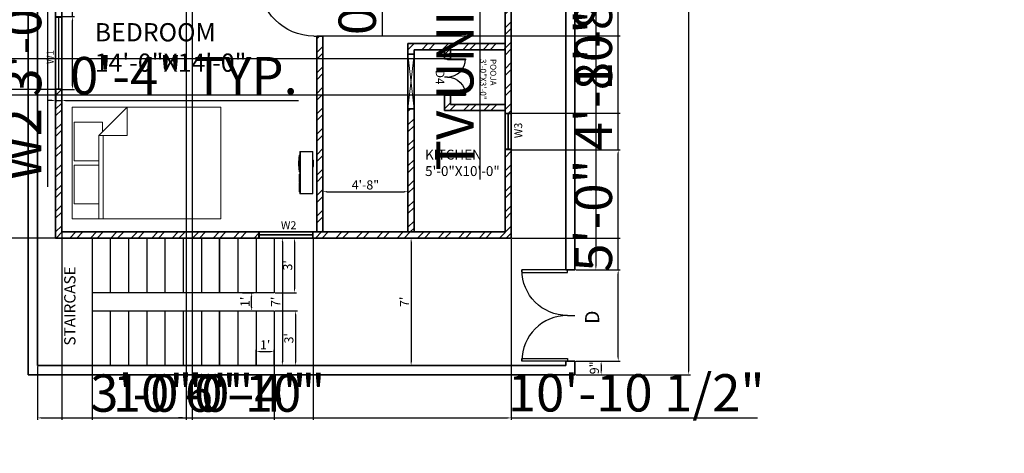
# Model space of a CAD drawing. Units: inches. Extents: x 1542 to 2523, y 1699 to 2449.
# Tile 2 of 7: x 1875 to 2523, y 1699 to 1984. Entities that reach past the tile are written whole.
import ezdxf

# ---------------------------------------------------------------- set-up
doc = ezdxf.new("R2010")
doc.units = ezdxf.units.IN
for name, color, linetype, lineweight in [('A-ANNO-DIMS', 7, 'Continuous', 18), ('A-ANNO-TEXT', 1, 'Continuous', 18), ('A-AREA-IDEN', 1, 'Continuous', 25), ('A-WALL-PATT', 9, 'Continuous', 13), ('doors', 5, 'Continuous', 25), ('furniture', 9, 'Continuous', 18), ('stair case', 6, 'Continuous', 25), ('walls', 7, 'Continuous', 35), ('windows', 93, 'Continuous', 18)]:
    doc.layers.add(name, color=color, linetype=linetype, lineweight=lineweight)
doc.styles.get("Standard").update_dxf_attribs({"font": 'arial.ttf'})
doc.dimstyles.new('ISO-25', dxfattribs={"dimtxt": 24.5625, "dimasz": 2.5, "dimexe": 1.25, "dimexo": 0.625, "dimtad": 1, "dimlunit": 4, "dimtxsty": 'Standard', "dimcen": 2.5, "dimadec": 0, "dimazin": 0, "dimtfac": 10, "dimtmove": 0, "dimatfit": 3, "dimfxl": 1, "dimarcsym": 0})

# ---------------------------------------------------------------- blocks, each defined once
blk = doc.blocks.new('*U2')
for p, q in [((0, 0), (0, -5)), ((30, 0), (30, -5))]:
    blk.add_line(p, q)
blk.add_lwpolyline([(0, 0), (0, 30), (1.75, 30), (1.75, 0)], close=True)
blk.add_arc((0, 0), 30, 0, 90)
blk = doc.blocks.new('Bed - Queen')
for p, q in [((0, -80.00003), (0, 0)), ((0, 0), (59.99999, 0)), ((59.99999, 0), (59.99999, -80.00003)), ((7.99999, -1.2), (28.79998, -1.2)), ((7.99999, -14.4), (7.99999, -1.2)), ((28.79998, -1.2), (28.79998, -14.4)), ((31.19999, -1.2), (51.99999, -1.2)), ((31.19999, -14.4), (31.19999, -1.2)), ((51.99999, -1.2), (51.99999, -16.4)), ((0, -14.4), (44.8, -14.4)), ((59.99999, -29.6), (44.8, -14.4)), ((44.8, -14.4), (44.8, -29.6)), ((44.8, -16.8), (0, -16.8)), ((51.99999, -16.4), (46.79936, -16.4)), ((44.8, -29.6), (59.99999, -29.6)), ((59.99999, -80.00003), (0, -80.00003))]:
    blk.add_line(p, q)
blk = doc.blocks.new('Entertainment Center')
for p, q in [((-4, 0), (-5, -1)), ((4, 0), (-4, 0)), ((5, -1), (4, 0)), ((-17, -19), (-17, -1)), ((-17, -1), (43, -1)), ((-16.5, -18.5), (-16.5, -1.5)), ((-16.5, -1.5), (42.5, -1.5)), ((42.5, -1.5), (42.5, -18.5)), ((43, -1), (43, -19)), ((43, -19), (-17, -19)), ((42.5, -18.5), (-16.5, -18.5)), ((-12, -20), (-12, -19)), ((12, -20), (-12, -20)), ((12, -19), (12, -20)), ((15, -20), (15, -19)), ((27, -20), (15, -20)), ((27, -19), (27, -20)), ((28, -20), (28, -19)), ((40, -20), (28, -20)), ((40, -19), (40, -20))]:
    blk.add_line(p, q)
blk.add_arc((0, 40), 61, 259.6111, 280.3889)
blk = doc.blocks.new('*D10')
at = {"layer": 'A-ANNO-DIMS', "color": 0, "lineweight": -2, "transparency": 16777216}
for p, q in [((2241.01, 2290.44), (2316.46, 2290.44)), ((2315.21, 2287.94), (2315.21, 1752.94)), ((2241.01, 1750.44), (2316.46, 1750.44))]:
    blk.add_line(p, q, dxfattribs=at)
at = {"layer": 'A-ANNO-DIMS', "color": 0, "transparency": 16777216}
for points in [[(2314.79, 2287.94), (2315.62, 2287.94), (2315.21, 2290.44)], [(2314.79, 1752.94), (2315.62, 1752.94), (2315.21, 1750.44)]]:
    blk.add_solid(points, dxfattribs=at)
at = {"layer": 'Defpoints', "color": 0, "transparency": 16777216}
for p in [(2240.38, 2290.44), (2240.38, 1750.44), (2315.21, 1750.44)]:
    blk.add_point(p, dxfattribs=at)
at = {"layer": 'A-ANNO-DIMS', "color": 0, "transparency": 16777216, "insert": (2308.48, 2020.44), "char_height": 12, "attachment_point": 5, "rotation": 90}
blk.add_mtext("45'", dxfattribs=at)
blk = doc.blocks.new('*D11')
at = {"layer": 'A-ANNO-DIMS', "color": 0, "lineweight": -2, "transparency": 16777216}
for p, q in [((2241.01, 2290.44), (2255.4, 2290.44)), ((2254.15, 2287.94), (2254.15, 1821.94)), ((2241.01, 1819.44), (2255.4, 1819.44))]:
    blk.add_line(p, q, dxfattribs=at)
at = {"layer": 'A-ANNO-DIMS', "color": 0, "transparency": 16777216}
for points in [[(2253.73, 2287.94), (2254.57, 2287.94), (2254.15, 2290.44)], [(2253.73, 1821.94), (2254.57, 1821.94), (2254.15, 1819.44)]]:
    blk.add_solid(points, dxfattribs=at)
at = {"layer": 'Defpoints', "color": 0, "transparency": 16777216}
for p in [(2240.38, 2290.44), (2240.38, 1819.44), (2254.15, 1819.44)]:
    blk.add_point(p, dxfattribs=at)
at = {"layer": 'A-ANNO-DIMS', "color": 0, "transparency": 16777216, "insert": (2250.46, 2054.94), "char_height": 6, "attachment_point": 5, "rotation": 90}
blk.add_mtext('39\'-3"', dxfattribs=at)
blk = doc.blocks.new('*D14')
at = {"layer": 'A-ANNO-DIMS', "color": 0, "lineweight": -2, "transparency": 16777216}
for p, q in [((2030.38, 1757.06), (2030.38, 1766.92)), ((2032.88, 1765.67), (2039.88, 1765.67)), ((2042.38, 1757.06), (2042.38, 1766.92))]:
    blk.add_line(p, q, dxfattribs=at)
at = {"layer": 'A-ANNO-DIMS', "color": 0, "transparency": 16777216}
for points in [[(2032.88, 1766.08), (2032.88, 1765.25), (2030.38, 1765.67)], [(2039.88, 1766.08), (2039.88, 1765.25), (2042.38, 1765.67)]]:
    blk.add_solid(points, dxfattribs=at)
at = {"layer": 'Defpoints', "color": 0, "transparency": 16777216}
for p in [(2042.38, 1765.67), (2030.38, 1756.44), (2042.38, 1756.44)]:
    blk.add_point(p, dxfattribs=at)
at = {"layer": 'A-ANNO-DIMS', "color": 0, "transparency": 16777216, "insert": (2036.38, 1769.3), "char_height": 6, "attachment_point": 5}
blk.add_mtext("1'", dxfattribs=at)
blk = doc.blocks.new('*D15')
at = {"layer": 'A-ANNO-DIMS', "color": 0, "lineweight": -2, "transparency": 16777216}
for p, q in [((2043.01, 1840.44), (2056.9, 1840.44)), ((2055.65, 1837.94), (2055.65, 1806.94)), ((2043.01, 1804.44), (2056.9, 1804.44))]:
    blk.add_line(p, q, dxfattribs=at)
at = {"layer": 'A-ANNO-DIMS', "color": 0, "transparency": 16777216}
for points in [[(2055.24, 1837.94), (2056.07, 1837.94), (2055.65, 1840.44)], [(2055.24, 1806.94), (2056.07, 1806.94), (2055.65, 1804.44)]]:
    blk.add_solid(points, dxfattribs=at)
at = {"layer": 'Defpoints', "color": 0, "transparency": 16777216}
for p in [(2042.38, 1840.44), (2042.38, 1804.44), (2055.65, 1804.44)]:
    blk.add_point(p, dxfattribs=at)
at = {"layer": 'A-ANNO-DIMS', "color": 0, "transparency": 16777216, "insert": (2051.96, 1822.44), "char_height": 6, "attachment_point": 5, "rotation": 90}
blk.add_mtext("3'", dxfattribs=at)
blk = doc.blocks.new('*D16')
at = {"layer": 'A-ANNO-DIMS', "color": 0, "lineweight": -2, "transparency": 16777216}
for p, q in [((2128.01, 1840.44), (2133.74, 1840.44)), ((2132.49, 1837.94), (2132.49, 1758.94)), ((2128.01, 1756.44), (2133.74, 1756.44))]:
    blk.add_line(p, q, dxfattribs=at)
at = {"layer": 'A-ANNO-DIMS', "color": 0, "transparency": 16777216}
for points in [[(2132.07, 1837.94), (2132.9, 1837.94), (2132.49, 1840.44)], [(2132.07, 1758.94), (2132.9, 1758.94), (2132.49, 1756.44)]]:
    blk.add_solid(points, dxfattribs=at)
at = {"layer": 'Defpoints', "color": 0, "transparency": 16777216}
for p in [(2127.38, 1840.44), (2127.38, 1756.44), (2132.49, 1756.44)]:
    blk.add_point(p, dxfattribs=at)
at = {"layer": 'A-ANNO-DIMS', "color": 0, "transparency": 16777216, "insert": (2128.86, 1798.44), "char_height": 6, "attachment_point": 5, "rotation": 90}
blk.add_mtext("7'", dxfattribs=at)
blk = doc.blocks.new('*D18')
at = {"layer": 'A-ANNO-DIMS', "color": 0, "lineweight": -2, "transparency": 16777216}
for p, q in [((2043.01, 1840.44), (2048.95, 1840.44)), ((2047.7, 1837.94), (2047.7, 1758.94)), ((2043.01, 1756.44), (2048.95, 1756.44))]:
    blk.add_line(p, q, dxfattribs=at)
at = {"layer": 'A-ANNO-DIMS', "color": 0, "transparency": 16777216}
for points in [[(2047.28, 1837.94), (2048.11, 1837.94), (2047.7, 1840.44)], [(2047.28, 1758.94), (2048.11, 1758.94), (2047.7, 1756.44)]]:
    blk.add_solid(points, dxfattribs=at)
at = {"layer": 'Defpoints', "color": 0, "transparency": 16777216}
for p in [(2042.38, 1840.44), (2042.38, 1756.44), (2047.7, 1756.44)]:
    blk.add_point(p, dxfattribs=at)
at = {"layer": 'A-ANNO-DIMS', "color": 0, "transparency": 16777216, "insert": (2044.07, 1798.44), "char_height": 6, "attachment_point": 5, "rotation": 90}
blk.add_mtext("7'", dxfattribs=at)
blk = doc.blocks.new('*D19')
at = {"layer": 'A-ANNO-DIMS', "color": 0, "lineweight": -2, "transparency": 16777216}
for p, q in [((2043.01, 1792.44), (2057.68, 1792.44)), ((2056.43, 1789.94), (2056.43, 1758.94)), ((2043.01, 1756.44), (2057.68, 1756.44))]:
    blk.add_line(p, q, dxfattribs=at)
at = {"layer": 'A-ANNO-DIMS', "color": 0, "transparency": 16777216}
for points in [[(2056.01, 1789.94), (2056.84, 1789.94), (2056.43, 1792.44)], [(2056.01, 1758.94), (2056.84, 1758.94), (2056.43, 1756.44)]]:
    blk.add_solid(points, dxfattribs=at)
at = {"layer": 'Defpoints', "color": 0, "transparency": 16777216}
for p in [(2042.38, 1792.44), (2042.38, 1756.44), (2056.43, 1756.44)]:
    blk.add_point(p, dxfattribs=at)
at = {"layer": 'A-ANNO-DIMS', "color": 0, "transparency": 16777216, "insert": (2052.74, 1774.44), "char_height": 6, "attachment_point": 5, "rotation": 90}
blk.add_mtext("3'", dxfattribs=at)
blk = doc.blocks.new('*D20')
at = {"layer": 'A-ANNO-DIMS', "color": 0, "lineweight": -2, "transparency": 16777216}
for p, q in [((2021.4, 1804.44), (2028.73, 1804.44)), ((2027.48, 1794.94), (2027.48, 1801.94)), ((2021.4, 1792.44), (2028.73, 1792.44))]:
    blk.add_line(p, q, dxfattribs=at)
at = {"layer": 'A-ANNO-DIMS', "color": 0, "transparency": 16777216}
for points in [[(2027.06, 1801.94), (2027.9, 1801.94), (2027.48, 1804.44)], [(2027.06, 1794.94), (2027.9, 1794.94), (2027.48, 1792.44)]]:
    blk.add_solid(points, dxfattribs=at)
at = {"layer": 'Defpoints', "color": 0, "transparency": 16777216}
for p in [(2020.78, 1804.44), (2027.48, 1804.44), (2020.78, 1792.44)]:
    blk.add_point(p, dxfattribs=at)
at = {"layer": 'A-ANNO-DIMS', "color": 0, "transparency": 16777216, "insert": (2023.84, 1798.44), "char_height": 6, "attachment_point": 5, "rotation": 90}
blk.add_mtext("1'", dxfattribs=at)
blk = doc.blocks.new('*D21')
at = {"layer": 'A-ANNO-DIMS', "color": 0, "lineweight": -2, "transparency": 16777216}
for p, q in [((2074.38, 1858.36), (2074.38, 1872.17)), ((2076.88, 1870.92), (2127.88, 1870.92)), ((2130.38, 1858.36), (2130.38, 1872.17))]:
    blk.add_line(p, q, dxfattribs=at)
at = {"layer": 'A-ANNO-DIMS', "color": 0, "transparency": 16777216}
for points in [[(2076.88, 1871.34), (2076.88, 1870.5), (2074.38, 1870.92)], [(2127.88, 1871.34), (2127.88, 1870.5), (2130.38, 1870.92)]]:
    blk.add_solid(points, dxfattribs=at)
at = {"layer": 'Defpoints', "color": 0, "transparency": 16777216}
for p in [(2130.38, 1870.92), (2074.38, 1857.74), (2130.38, 1857.74)]:
    blk.add_point(p, dxfattribs=at)
at = {"layer": 'A-ANNO-DIMS', "color": 0, "transparency": 16777216, "insert": (2102.38, 1874.61), "char_height": 6, "attachment_point": 5}
blk.add_mtext('4\'-8"', dxfattribs=at)
blk = doc.blocks.new('*D22')
at = {"layer": 'A-ANNO-DIMS', "color": 0, "lineweight": -2, "transparency": 16777216}
for p, q in [((2241.01, 1759.44), (2258.85, 1759.44)), ((2257.6, 1756.94), (2257.6, 1752.94)), ((2241.01, 1750.44), (2258.85, 1750.44))]:
    blk.add_line(p, q, dxfattribs=at)
at = {"layer": 'A-ANNO-DIMS', "color": 0, "transparency": 16777216}
for points in [[(2257.18, 1756.94), (2258.02, 1756.94), (2257.6, 1759.44)], [(2257.18, 1752.94), (2258.02, 1752.94), (2257.6, 1750.44)]]:
    blk.add_solid(points, dxfattribs=at)
at = {"layer": 'Defpoints', "color": 0, "transparency": 16777216}
for p in [(2240.38, 1759.44), (2240.38, 1750.44), (2257.6, 1750.44)]:
    blk.add_point(p, dxfattribs=at)
at = {"layer": 'A-ANNO-DIMS', "color": 0, "transparency": 16777216, "insert": (2253.91, 1754.94), "char_height": 6, "attachment_point": 5, "rotation": 90}
blk.add_mtext('9"', dxfattribs=at)
blk = doc.blocks.new('WIN-W3-24IN')
for p, q in [((0, 0), (0, 24.03)), ((0, 24.03), (3.94, 24.03)), ((0, 23.53), (3.94, 23.53)), ((1.77, 0.5), (1.77, 23.53)), ((2.17, 0.5), (2.17, 23.53)), ((3.94, 24.03), (3.94, 0)), ((3.94, 0.5), (0, 0.5)), ((3.94, 0), (0, 0))]:
    blk.add_line(p, q)
blk = doc.blocks.new('WIN-W2-36IN')
for p, q in [((0, 3.94), (36.03, 3.94)), ((0, 0), (0, 3.94)), ((36.03, 0), (0, 0)), ((0.5, 0), (0.5, 3.94)), ((0.5, 2.17), (35.53, 2.17)), ((0.5, 1.77), (35.53, 1.77)), ((35.53, 3.94), (35.53, 0)), ((36.03, 3.94), (36.03, 0))]:
    blk.add_line(p, q)
blk = doc.blocks.new('WIN-W1-48IN')
for p, q in [((0, 0), (0, 48.03)), ((0, 48.03), (3.94, 48.03)), ((0, 47.53), (3.94, 47.53)), ((1.77, 0.5), (1.77, 47.53)), ((2.17, 0.5), (2.17, 47.53)), ((3.94, 48.03), (3.94, 0)), ((3.94, 0.5), (0, 0.5)), ((3.94, 0), (0, 0))]:
    blk.add_line(p, q)
blk = doc.blocks.new('*D27')
at = {"layer": 'A-ANNO-DIMS', "color": 0, "lineweight": -2, "transparency": 16777216}
for p, q in [((2114.72, 2156.7), (2112.11, 2156.7)), ((2113.36, 2154.2), (2113.36, 2148.3)), ((2114.72, 2145.8), (2112.11, 2145.8)), ((2113.36, 2145.8), (2113.36, 1973.25))]:
    blk.add_line(p, q, dxfattribs=at)
at = {"layer": 'A-ANNO-DIMS', "color": 0, "transparency": 16777216}
for points in [[(2112.94, 2154.2), (2113.78, 2154.2), (2113.36, 2156.7)], [(2112.94, 2148.3), (2113.78, 2148.3), (2113.36, 2145.8)]]:
    blk.add_solid(points, dxfattribs=at)
at = {"layer": 'Defpoints', "color": 0, "transparency": 16777216}
for p in [(2115.34, 2156.7), (2113.36, 2145.8), (2115.34, 2145.8)]:
    blk.add_point(p, dxfattribs=at)
at = {"layer": 'A-ANNO-DIMS', "color": 0, "transparency": 16777216, "insert": (2100.19, 2058.28), "char_height": 24.5625, "attachment_point": 5, "rotation": 90}
blk.add_mtext('0\'-11" TYP.', dxfattribs=at)
blk = doc.blocks.new('*D30')
at = {"layer": 'A-ANNO-DIMS', "color": 0, "lineweight": -2, "transparency": 16777216}
for p, q in [((2181.19, 2203.89), (2176.38, 2203.89)), ((2177.63, 2201.39), (2177.63, 2178.49)), ((2181.19, 2175.99), (2176.38, 2175.99)), ((2177.63, 2175.99), (2177.63, 1878.93))]:
    blk.add_line(p, q, dxfattribs=at)
at = {"layer": 'A-ANNO-DIMS', "color": 0, "transparency": 16777216}
for points in [[(2177.21, 2201.39), (2178.05, 2201.39), (2177.63, 2203.89)], [(2177.21, 2178.49), (2178.05, 2178.49), (2177.63, 2175.99)]]:
    blk.add_solid(points, dxfattribs=at)
at = {"layer": 'Defpoints', "color": 0, "transparency": 16777216}
for p in [(2181.81, 2203.89), (2177.63, 2175.99), (2181.81, 2175.99)]:
    blk.add_point(p, dxfattribs=at)
at = {"layer": 'A-ANNO-DIMS', "color": 0, "transparency": 16777216, "insert": (2164.46, 2026.21), "char_height": 24.5625, "attachment_point": 5, "rotation": 90}
blk.add_mtext('TV UNIT 2\'-4" TYP.', dxfattribs=at)
blk = doc.blocks.new('*D36')
at = {"layer": 'A-ANNO-DIMS', "color": 0, "lineweight": -2, "transparency": 16777216}
for p, q in [((1897.82, 2125.68), (1891.79, 2125.68)), ((1893.04, 2123.18), (1893.04, 2092.15)), ((1897.82, 2089.65), (1891.79, 2089.65)), ((1893.04, 2089.65), (1893.04, 1874.17))]:
    blk.add_line(p, q, dxfattribs=at)
at = {"layer": 'A-ANNO-DIMS', "color": 0, "transparency": 16777216}
for points in [[(1892.62, 2123.18), (1893.46, 2123.18), (1893.04, 2125.68)], [(1892.62, 2092.15), (1893.46, 2092.15), (1893.04, 2089.65)]]:
    blk.add_solid(points, dxfattribs=at)
at = {"layer": 'Defpoints', "color": 0, "transparency": 16777216}
for p in [(1898.45, 2125.68), (1893.04, 2089.65), (1898.45, 2089.65)]:
    blk.add_point(p, dxfattribs=at)
at = {"layer": 'A-ANNO-DIMS', "color": 0, "transparency": 16777216, "insert": (1879.87, 1980.66), "char_height": 24.5625, "attachment_point": 5, "rotation": 90}
blk.add_mtext('W2 3\'-0" TYP.', dxfattribs=at)
blk = doc.blocks.new('*D40')
at = {"layer": 'A-ANNO-DIMS', "color": 0, "lineweight": -2, "transparency": 16777216}
for p, q in [((1909.59, 1986.22), (1909.59, 2201.7)), ((1903.01, 1986.22), (1910.84, 1986.22)), ((1909.59, 1940.69), (1909.59, 1983.72)), ((1903.01, 1938.19), (1910.84, 1938.19))]:
    blk.add_line(p, q, dxfattribs=at)
at = {"layer": 'A-ANNO-DIMS', "color": 0, "transparency": 16777216}
for points in [[(1909.17, 1983.72), (1910, 1983.72), (1909.59, 1986.22)], [(1909.17, 1940.69), (1910, 1940.69), (1909.59, 1938.19)]]:
    blk.add_solid(points, dxfattribs=at)
at = {"layer": 'Defpoints', "color": 0, "transparency": 16777216}
for p in [(1902.38, 1986.22), (1909.59, 1986.22), (1902.38, 1938.19)]:
    blk.add_point(p, dxfattribs=at)
at = {"layer": 'A-ANNO-DIMS', "color": 0, "transparency": 16777216, "insert": (1896.42, 2095.21), "char_height": 24.5625, "attachment_point": 5, "rotation": 90}
blk.add_mtext('W1 4\'-0" TYP.', dxfattribs=at)
blk = doc.blocks.new('*D41')
at = {"layer": 'A-ANNO-DIMS', "color": 0, "lineweight": -2, "transparency": 16777216}
for p, q in [((1898.45, 1937.57), (1898.45, 1929.74)), ((1902.38, 1937.57), (1902.38, 1929.74)), ((1895.95, 1930.99), (1893.45, 1930.99)), ((1898.45, 1930.99), (1902.38, 1930.99)), ((1904.88, 1930.99), (2058.35, 1930.99))]:
    blk.add_line(p, q, dxfattribs=at)
at = {"layer": 'A-ANNO-DIMS', "color": 0, "transparency": 16777216}
for points in [[(1895.95, 1931.4), (1895.95, 1930.57), (1898.45, 1930.99)], [(1904.88, 1931.4), (1904.88, 1930.57), (1902.38, 1930.99)]]:
    blk.add_solid(points, dxfattribs=at)
at = {"layer": 'Defpoints', "color": 0, "transparency": 16777216}
for p in [(1898.45, 1938.19), (1902.38, 1938.19), (1902.38, 1930.99)]:
    blk.add_point(p, dxfattribs=at)
at = {"layer": 'A-ANNO-DIMS', "color": 0, "transparency": 16777216, "insert": (1982.87, 1944.15), "char_height": 24.562, "attachment_point": 5}
blk.add_mtext('0\'-4" TYP.', dxfattribs=at)
blk = doc.blocks.new('*D42')
at = {"layer": 'A-ANNO-DIMS', "color": 0, "lineweight": -2, "transparency": 16777216}
for p, q in [((2131.75, 2027.78), (2131.75, 2037.46)), ((2134.25, 2036.21), (2189.62, 2036.21)), ((2192.12, 2027.78), (2192.12, 2037.46)), ((2192.12, 2036.21), (2523.07, 2036.21))]:
    blk.add_line(p, q, dxfattribs=at)
at = {"layer": 'A-ANNO-DIMS', "color": 0, "transparency": 16777216}
for points in [[(2134.25, 2036.63), (2134.25, 2035.8), (2131.75, 2036.21)], [(2189.62, 2036.63), (2189.62, 2035.8), (2192.12, 2036.21)]]:
    blk.add_solid(points, dxfattribs=at)
at = {"layer": 'Defpoints', "color": 0, "transparency": 16777216}
for p in [(2192.12, 2036.21), (2131.75, 2027.16), (2192.12, 2027.16)]:
    blk.add_point(p, dxfattribs=at)
at = {"layer": 'A-ANNO-DIMS', "color": 0, "transparency": 16777216, "insert": (2358.84, 2049.54), "char_height": 24.5625, "attachment_point": 5}
blk.add_mtext('DINING SET 5\'-0 1/2"', dxfattribs=at)
blk = doc.blocks.new('*D47')
at = {"layer": 'A-ANNO-DIMS', "color": 0, "lineweight": -2, "transparency": 16777216}
for p, q in [((2268.83, 2009.44), (2268.83, 2078.47)), ((2071.01, 2009.44), (2270.08, 2009.44)), ((2268.83, 1975.94), (2268.83, 2006.94)), ((2071.01, 1973.44), (2270.08, 1973.44))]:
    blk.add_line(p, q, dxfattribs=at)
at = {"layer": 'A-ANNO-DIMS', "color": 0, "transparency": 16777216}
for points in [[(2268.42, 2006.94), (2269.25, 2006.94), (2268.83, 2009.44)], [(2268.42, 1975.94), (2269.25, 1975.94), (2268.83, 1973.44)]]:
    blk.add_solid(points, dxfattribs=at)
at = {"layer": 'Defpoints', "color": 0, "transparency": 16777216}
for p in [(2070.38, 2009.44), (2268.83, 2009.44), (2070.38, 1973.44)]:
    blk.add_point(p, dxfattribs=at)
at = {"layer": 'A-ANNO-DIMS', "color": 0, "transparency": 16777216, "insert": (2255.66, 2045.2), "char_height": 24.562, "attachment_point": 5, "rotation": 90}
blk.add_mtext('3\'-0"', dxfattribs=at)
blk = doc.blocks.new('*D49')
at = {"layer": 'A-ANNO-DIMS', "color": 0, "lineweight": -2, "transparency": 16777216}
for p, q in [((1851.93, 1958.44), (1851.93, 2027.9)), ((2157.76, 1958.44), (1850.68, 1958.44)), ((1851.93, 1936.94), (1851.93, 1955.94)), ((2157.76, 1934.44), (1850.68, 1934.44))]:
    blk.add_line(p, q, dxfattribs=at)
at = {"layer": 'A-ANNO-DIMS', "color": 0, "transparency": 16777216}
for points in [[(1851.52, 1955.94), (1852.35, 1955.94), (1851.93, 1958.44)], [(1851.52, 1936.94), (1852.35, 1936.94), (1851.93, 1934.44)]]:
    blk.add_solid(points, dxfattribs=at)
at = {"layer": 'Defpoints', "color": 0, "transparency": 16777216}
for p in [(1851.93, 1958.44), (2158.38, 1958.44), (2158.38, 1934.44)]:
    blk.add_point(p, dxfattribs=at)
at = {"layer": 'A-ANNO-DIMS', "color": 0, "transparency": 16777216, "insert": (1838.77, 1994.42), "char_height": 24.562, "attachment_point": 5, "rotation": 90}
blk.add_mtext('2\'-0"', dxfattribs=at)
blk = doc.blocks.new('*D51')
at = {"layer": 'A-ANNO-DIMS', "color": 0, "lineweight": -2, "transparency": 16777216}
for p, q in [((2268.83, 1819.44), (2268.83, 1888.48)), ((2241.01, 1819.44), (2270.08, 1819.44)), ((2268.83, 1761.94), (2268.83, 1816.94)), ((2241.01, 1759.44), (2270.08, 1759.44))]:
    blk.add_line(p, q, dxfattribs=at)
at = {"layer": 'A-ANNO-DIMS', "color": 0, "transparency": 16777216}
for points in [[(2268.42, 1816.94), (2269.25, 1816.94), (2268.83, 1819.44)], [(2268.42, 1761.94), (2269.25, 1761.94), (2268.83, 1759.44)]]:
    blk.add_solid(points, dxfattribs=at)
at = {"layer": 'Defpoints', "color": 0, "transparency": 16777216}
for p in [(2240.38, 1819.44), (2268.83, 1819.44), (2240.38, 1759.44)]:
    blk.add_point(p, dxfattribs=at)
at = {"layer": 'A-ANNO-DIMS', "color": 0, "transparency": 16777216, "insert": (2255.67, 1855.21), "char_height": 24.562, "attachment_point": 5, "rotation": 90}
blk.add_mtext('5\'-0"', dxfattribs=at)
blk = doc.blocks.new('*D52')
at = {"layer": 'A-ANNO-DIMS', "color": 0, "lineweight": -2, "transparency": 16777216}
for p, q in [((1886.38, 1755.81), (1886.38, 1720.74)), ((1922.38, 1755.81), (1922.38, 1720.74)), ((1888.88, 1721.99), (1919.88, 1721.99)), ((1922.38, 1721.99), (1991.41, 1721.99))]:
    blk.add_line(p, q, dxfattribs=at)
at = {"layer": 'A-ANNO-DIMS', "color": 0, "transparency": 16777216}
for points in [[(1888.88, 1722.41), (1888.88, 1721.57), (1886.38, 1721.99)], [(1919.88, 1722.41), (1919.88, 1721.57), (1922.38, 1721.99)]]:
    blk.add_solid(points, dxfattribs=at)
at = {"layer": 'Defpoints', "color": 0, "transparency": 16777216}
for p in [(1886.38, 1756.44), (1922.38, 1756.44), (1922.38, 1721.99)]:
    blk.add_point(p, dxfattribs=at)
at = {"layer": 'A-ANNO-DIMS', "color": 0, "transparency": 16777216, "insert": (1958.15, 1735.16), "char_height": 24.562, "attachment_point": 5}
blk.add_mtext('3\'-0"', dxfattribs=at)
blk = doc.blocks.new('*D53')
at = {"layer": 'A-ANNO-DIMS', "color": 0, "lineweight": -2, "transparency": 16777216}
for p, q in [((1922.38, 1755.81), (1922.38, 1720.74)), ((2042.38, 1755.81), (2042.38, 1720.74)), ((1924.88, 1721.99), (2039.88, 1721.99))]:
    blk.add_line(p, q, dxfattribs=at)
at = {"layer": 'A-ANNO-DIMS', "color": 0, "transparency": 16777216}
for points in [[(1924.88, 1722.41), (1924.88, 1721.57), (1922.38, 1721.99)], [(2039.88, 1722.41), (2039.88, 1721.57), (2042.38, 1721.99)]]:
    blk.add_solid(points, dxfattribs=at)
at = {"layer": 'Defpoints', "color": 0, "transparency": 16777216}
for p in [(1922.38, 1756.44), (2042.38, 1756.44), (2042.38, 1721.99)]:
    blk.add_point(p, dxfattribs=at)
at = {"layer": 'A-ANNO-DIMS', "color": 0, "transparency": 16777216, "insert": (1982.38, 1735.15), "char_height": 24.562, "attachment_point": 5}
blk.add_mtext('10\'-0"', dxfattribs=at)
blk = doc.blocks.new('*D55')
at = {"layer": 'A-ANNO-DIMS', "color": 0, "lineweight": -2, "transparency": 16777216}
for p, q in [((1897.82, 1938.19), (1850.68, 1938.19)), ((1851.93, 1842.94), (1851.93, 1935.69)), ((1897.76, 1840.44), (1850.68, 1840.44))]:
    blk.add_line(p, q, dxfattribs=at)
at = {"layer": 'A-ANNO-DIMS', "color": 0, "transparency": 16777216}
for points in [[(1851.52, 1935.69), (1852.35, 1935.69), (1851.93, 1938.19)], [(1851.52, 1842.94), (1852.35, 1842.94), (1851.93, 1840.44)]]:
    blk.add_solid(points, dxfattribs=at)
at = {"layer": 'Defpoints', "color": 0, "transparency": 16777216}
for p in [(1851.93, 1938.19), (1898.45, 1938.19), (1898.38, 1840.44)]:
    blk.add_point(p, dxfattribs=at)
at = {"layer": 'A-ANNO-DIMS', "color": 0, "transparency": 16777216, "insert": (1838.77, 1889.31), "char_height": 24.562, "attachment_point": 5, "rotation": 90}
blk.add_mtext('8\'-2"', dxfattribs=at)
blk = doc.blocks.new('*D58')
at = {"layer": 'A-ANNO-DIMS', "color": 0, "lineweight": -2, "transparency": 16777216}
for p, q in [((2268.83, 1898.59), (2268.83, 1987.71)), ((2199.01, 1898.59), (2270.08, 1898.59)), ((2268.83, 1842.94), (2268.83, 1896.09)), ((2199.01, 1840.44), (2270.08, 1840.44))]:
    blk.add_line(p, q, dxfattribs=at)
at = {"layer": 'A-ANNO-DIMS', "color": 0, "transparency": 16777216}
for points in [[(2268.42, 1896.09), (2269.25, 1896.09), (2268.83, 1898.59)], [(2268.42, 1842.94), (2269.25, 1842.94), (2268.83, 1840.44)]]:
    blk.add_solid(points, dxfattribs=at)
at = {"layer": 'Defpoints', "color": 0, "transparency": 16777216}
for p in [(2198.38, 1898.59), (2268.83, 1898.59), (2198.38, 1840.44)]:
    blk.add_point(p, dxfattribs=at)
at = {"layer": 'A-ANNO-DIMS', "color": 0, "transparency": 16777216, "insert": (2255.67, 1944.4), "char_height": 24.562, "attachment_point": 5, "rotation": 90}
blk.add_mtext('4\'-10"', dxfattribs=at)
blk = doc.blocks.new('*D59')
at = {"layer": 'A-ANNO-DIMS', "color": 0, "lineweight": -2, "transparency": 16777216}
for p, q in [((2199.01, 2026.86), (2270.08, 2026.86)), ((2268.83, 1925.12), (2268.83, 2024.36)), ((2199.01, 1922.62), (2270.08, 1922.62))]:
    blk.add_line(p, q, dxfattribs=at)
at = {"layer": 'A-ANNO-DIMS', "color": 0, "transparency": 16777216}
for points in [[(2268.42, 2024.36), (2269.25, 2024.36), (2268.83, 2026.86)], [(2268.42, 1925.12), (2269.25, 1925.12), (2268.83, 1922.62)]]:
    blk.add_solid(points, dxfattribs=at)
at = {"layer": 'Defpoints', "color": 0, "transparency": 16777216}
for p in [(2198.38, 2026.86), (2268.83, 2026.86), (2198.38, 1922.62)]:
    blk.add_point(p, dxfattribs=at)
at = {"layer": 'A-ANNO-DIMS', "color": 0, "transparency": 16777216, "insert": (2255.67, 1974.74), "char_height": 24.562, "attachment_point": 5, "rotation": 90}
blk.add_mtext('8\'-8"', dxfattribs=at)
blk = doc.blocks.new('*D64')
at = {"layer": 'A-ANNO-DIMS', "color": 0, "lineweight": -2, "transparency": 16777216}
for p, q in [((2068.07, 1839.88), (2068.07, 1720.74)), ((2198.38, 1839.81), (2198.38, 1720.74)), ((2070.57, 1721.99), (2195.88, 1721.99)), ((2198.38, 1721.99), (2360.52, 1721.99))]:
    blk.add_line(p, q, dxfattribs=at)
at = {"layer": 'A-ANNO-DIMS', "color": 0, "transparency": 16777216}
for points in [[(2070.57, 1722.41), (2070.57, 1721.57), (2068.07, 1721.99)], [(2195.88, 1722.41), (2195.88, 1721.57), (2198.38, 1721.99)]]:
    blk.add_solid(points, dxfattribs=at)
at = {"layer": 'Defpoints', "color": 0, "transparency": 16777216}
for p in [(2068.07, 1840.5), (2198.38, 1840.44), (2198.38, 1721.99)]:
    blk.add_point(p, dxfattribs=at)
at = {"layer": 'A-ANNO-DIMS', "color": 0, "transparency": 16777216, "insert": (2280.7, 1735.31), "char_height": 24.5625, "attachment_point": 5}
blk.add_mtext('10\'-10 1/2"', dxfattribs=at)
blk = doc.blocks.new('*D67')
at = {"layer": 'A-ANNO-DIMS', "color": 0, "lineweight": -2, "transparency": 16777216}
for p, q in [((1902.38, 2011.81), (1902.38, 1720.74)), ((1984.38, 2015.81), (1984.38, 1720.74)), ((1904.88, 1721.99), (1981.88, 1721.99)), ((1984.38, 1721.99), (2072.64, 1721.99))]:
    blk.add_line(p, q, dxfattribs=at)
at = {"layer": 'A-ANNO-DIMS', "color": 0, "transparency": 16777216}
for points in [[(1904.88, 1722.41), (1904.88, 1721.57), (1902.38, 1721.99)], [(1981.88, 1722.41), (1981.88, 1721.57), (1984.38, 1721.99)]]:
    blk.add_solid(points, dxfattribs=at)
at = {"layer": 'Defpoints', "color": 0, "transparency": 16777216}
for p in [(1984.38, 2016.44), (1902.38, 2012.44), (1984.38, 1721.99)]:
    blk.add_point(p, dxfattribs=at)
at = {"layer": 'A-ANNO-DIMS', "color": 0, "transparency": 16777216, "insert": (2029.76, 1735.15), "char_height": 24.562, "attachment_point": 5}
blk.add_mtext('6\'-10"', dxfattribs=at)
blk = doc.blocks.new('*D68')
at = {"layer": 'A-ANNO-DIMS', "color": 0, "lineweight": -2, "transparency": 16777216}
for p, q in [((1984.38, 2015.81), (1984.38, 1720.74)), ((1988.38, 2015.81), (1988.38, 1720.74)), ((1981.88, 1721.99), (1979.38, 1721.99)), ((1984.38, 1721.99), (1988.38, 1721.99)), ((1990.88, 1721.99), (2059.93, 1721.99))]:
    blk.add_line(p, q, dxfattribs=at)
at = {"layer": 'A-ANNO-DIMS', "color": 0, "transparency": 16777216}
for points in [[(1981.88, 1722.41), (1981.88, 1721.57), (1984.38, 1721.99)], [(1990.88, 1722.41), (1990.88, 1721.57), (1988.38, 1721.99)]]:
    blk.add_solid(points, dxfattribs=at)
at = {"layer": 'Defpoints', "color": 0, "transparency": 16777216}
for p in [(1984.38, 2016.44), (1988.38, 2016.44), (1988.38, 1721.99)]:
    blk.add_point(p, dxfattribs=at)
at = {"layer": 'A-ANNO-DIMS', "color": 0, "transparency": 16777216, "insert": (2026.65, 1735.15), "char_height": 24.562, "attachment_point": 5}
blk.add_mtext('0\'-4"', dxfattribs=at)

msp = doc.modelspace()

# ---------------------------------------------------------------- hatches: boundary and pattern name
at = {"layer": 'A-WALL-PATT'}
h = msp.add_hatch(dxfattribs=at)
h.set_pattern_fill('ANSI32', color=256)
h.paths.add_polyline_path([(2198.383, 2026.862), (2194.383, 2026.862), (2194.383, 1922.623), (2198.383, 1922.623)])
h = msp.add_hatch(dxfattribs=at)
h.set_pattern_fill('ANSI32', color=256)
h.paths.add_polyline_path([(2074.383, 1973.439), (2070.383, 1973.439), (2070.383, 1844.439), (2074.383, 1844.439)])
h = msp.add_hatch(dxfattribs=at)
h.set_pattern_fill('ANSI32', color=256)
h.paths.add_polyline_path([(2194.383, 1968.439), (2130.383, 1968.439), (2130.383, 1961.439), (2134.383, 1961.439), (2134.383, 1964.439), (2194.383, 1964.439)])
h = msp.add_hatch(dxfattribs=at)
h.set_pattern_fill('ANSI32', color=256)
h.paths.add_polyline_path([(2158.383, 1964.439), (2154.383, 1964.439), (2154.383, 1958.439), (2156.383, 1958.439), (2158.383, 1958.439)])
h = msp.add_hatch(dxfattribs=at)
h.set_pattern_fill('ANSI32', color=256)
h.paths.add_polyline_path([(2032.035, 1844.439), (1902.383, 1844.439), (1902.383, 1938.191), (1898.383, 1938.191), (1898.383, 1840.439), (2032.035, 1840.439)])
h = msp.add_hatch(dxfattribs=at)
h.set_pattern_fill('ANSI32', color=256)
h.paths.add_polyline_path([(2194.383, 1928.439), (2158.383, 1928.439), (2158.383, 1934.439), (2156.383, 1934.439), (2154.383, 1934.439), (2154.383, 1924.439), (2194.383, 1924.439)])
h = msp.add_hatch(dxfattribs=at)
h.set_pattern_fill('ANSI32', color=256)
h.paths.add_polyline_path([(2134.383, 1925.439), (2130.383, 1925.439), (2130.383, 1844.439), (2134.383, 1844.439)])
h = msp.add_hatch(dxfattribs=at)
h.set_pattern_fill('ANSI32', color=256)
h.paths.add_polyline_path([(2198.383, 1898.591), (2194.383, 1898.591), (2194.383, 1844.439), (2127.383, 1844.439), (2068.067, 1844.439), (2068.067, 1840.439), (2127.383, 1840.439), (2198.383, 1840.439)])

# ---------------------------------------------------------------- linework, layer by layer
at = {"layer": 'stair case'}
for p, q in [((2006.383, 1840.439), (1886.383, 1840.439)), ((1886.383, 1840.439), (1886.383, 1756.439)), ((1922.383, 1840.439), (1922.383, 1756.439)), ((1934.383, 1840.439), (1934.383, 1804.439)), ((1946.383, 1840.439), (1946.383, 1804.439)), ((1958.383, 1840.439), (1958.383, 1804.439)), ((1970.383, 1840.439), (1970.383, 1804.439)), ((1982.383, 1840.439), (1982.383, 1804.439)), ((1994.383, 1840.439), (1994.383, 1804.439)), ((2006.383, 1840.439), (2006.383, 1804.439)), ((2006.383, 1840.439), (2042.383, 1840.439)), ((2006.383, 1804.439), (2006.383, 1840.439)), ((2018.383, 1840.439), (2018.383, 1804.439)), ((2030.383, 1840.439), (2030.383, 1804.439)), ((2042.383, 1840.439), (2042.383, 1804.439)), ((2042.383, 1804.439), (1922.383, 1804.439)), ((1922.383, 1792.439), (2042.383, 1792.439)), ((1934.383, 1792.439), (1934.383, 1756.439)), ((1946.383, 1792.439), (1946.383, 1756.439)), ((1958.383, 1792.439), (1958.383, 1756.439)), ((1970.383, 1792.439), (1970.383, 1756.439)), ((1982.383, 1792.439), (1982.383, 1756.439)), ((1994.383, 1792.439), (1994.383, 1756.439)), ((2006.383, 1756.439), (2006.383, 1792.439)), ((2006.383, 1792.439), (2006.383, 1756.439)), ((2018.383, 1792.439), (2018.383, 1756.439)), ((2030.383, 1792.439), (2030.383, 1756.439)), ((2042.383, 1792.439), (2042.383, 1756.439)), ((1886.383, 1756.439), (2006.383, 1756.439)), ((2006.383, 1756.439), (2042.383, 1756.439))]:
    msp.add_line(p, q, dxfattribs=at)
at = {"layer": 'walls'}
for p, q in [((1880.383, 1750.439), (1880.383, 2290.439)), ((2240.383, 2290.439), (2240.383, 1819.439)), ((1886.383, 1756.439), (1886.383, 2284.439)), ((2234.383, 2284.439), (2234.383, 1819.439)), ((1898.383, 1840.439), (1898.383, 2252.439)), ((1902.383, 1844.439), (1902.383, 2248.439)), ((2194.383, 2083.439), (2194.383, 1844.439)), ((2198.383, 2083.439), (2198.383, 1840.439)), ((2070.383, 1844.439), (2070.383, 1973.439)), ((2070.383, 1973.439), (2074.383, 1973.439)), ((2074.383, 1844.439), (2074.383, 1973.439)), ((2130.383, 1968.439), (2130.383, 1961.439)), ((2194.383, 1968.439), (2130.383, 1968.439)), ((2134.383, 1961.439), (2130.383, 1961.439)), ((2130.383, 1961.439), (2130.383, 1844.439)), ((2134.383, 1964.439), (2134.383, 1961.439)), ((2194.383, 1964.439), (2134.383, 1964.439)), ((2134.383, 1964.439), (2134.383, 1961.439)), ((2134.383, 1961.439), (2134.383, 1844.439)), ((2154.383, 1964.439), (2154.383, 1958.439)), ((2158.383, 1958.439), (2154.383, 1958.439)), ((2158.383, 1964.439), (2158.383, 1958.439)), ((2158.383, 1964.439), (2158.383, 1958.439)), ((2154.383, 1934.439), (2158.383, 1934.439)), ((2154.383, 1934.439), (2154.383, 1924.439)), ((2158.383, 1934.439), (2158.383, 1928.439)), ((2194.383, 1928.439), (2158.383, 1928.439)), ((2130.383, 1925.439), (2134.383, 1925.439)), ((2134.383, 1925.439), (2130.383, 1925.439)), ((2194.383, 1924.439), (2154.383, 1924.439)), ((2127.383, 1844.439), (1902.383, 1844.439)), ((2194.383, 1844.439), (2127.383, 1844.439)), ((2130.383, 1844.439), (2127.383, 1844.439)), ((2127.383, 1840.439), (1898.383, 1840.439)), ((2198.383, 1840.439), (2127.383, 1840.439)), ((2240.383, 1819.439), (2234.383, 1819.439)), ((2234.383, 1756.439), (2234.383, 1759.439)), ((2234.383, 1759.439), (2240.383, 1759.439)), ((2234.383, 1759.439), (2234.383, 1756.439)), ((2240.383, 1759.439), (2240.383, 1750.439)), ((2234.383, 1756.439), (1886.383, 1756.439)), ((2240.383, 1750.439), (1880.383, 1750.439))]:
    msp.add_line(p, q, dxfattribs=at)
at = {"layer": 'windows'}
for p, q in [((2130.383, 1925.439), (2134.383, 1961.439)), ((2130.383, 1961.439), (2134.383, 1925.439))]:
    msp.add_line(p, q, dxfattribs=at)

# ---------------------------------------------------------------- block references
at = {"layer": 'doors'}
for p, xscale, yscale, zscale, rotation in [((2068.383, 2009.439), -1.199999999999999, 1.199999999999999, 1.199999999999999, 90), ((2156.383, 1958.439), 0.4, 0.4, 0.4, 270), ((2156.383, 1934.439), -0.4, 0.4, 0.4, 270)]:
    msp.add_blockref('*U2', p, dxfattribs=dict(at, xscale=xscale, yscale=yscale, zscale=zscale, rotation=rotation))
at = {"layer": 'doors', "xscale": -1, "rotation": 90}
msp.add_blockref('*U2', (2235.383, 1819.439), dxfattribs=at)
at = {"layer": 'doors', "rotation": 90}
msp.add_blockref('*U2', (2235.383, 1759.439), dxfattribs=at)
at = {"layer": 'furniture'}
for name, p, xscale, yscale, zscale, rotation in [('Bed - Queen', (1909.25, 1853.156), 1.223193858347369, 1.223193858347369, 1.223193858347369, 90), ('Entertainment Center', (2068.134, 1889.508), 0.4648726153281338, 0.4648726153281338, 0.4648726153281338, 270)]:
    msp.add_blockref(name, p, dxfattribs=dict(at, xscale=xscale, yscale=yscale, zscale=zscale, rotation=rotation))
at = {"layer": 'windows'}
for name, p in [('WIN-W1-48IN', (1898.446, 1938.191)), ('WIN-W2-36IN', (2032.035, 1840.502))]:
    msp.add_blockref(name, p, dxfattribs=at)
at = {"layer": 'windows', "rotation": 180}
msp.add_blockref('WIN-W3-24IN', (2198.383, 1922.624), dxfattribs=at)

# ---------------------------------------------------------------- texts
at = {"layer": 'A-ANNO-TEXT', "attachment_point": 1}
for s, width, gutter_width, insert, char_height, rotation in [('W1', 1.45099, 23.402, (1892.505, 1954.993), 4.6805, 90), ('D4', 5.66597, 28.33, (2154.383, 1951.103), 5.666, 270), ('W3', 1.62225, 26.164, (2200.387, 1906.127), 5.2329, 90), ('D', 3.38383, 46.636, (2247.016, 1783.919), 9.327, 90)]:
    msp.add_mtext_dynamic_manual_height_columns(s, width=width, gutter_width=gutter_width, heights=[0], dxfattribs=dict(at, insert=insert, char_height=char_height, rotation=rotation))
at = {"layer": 'A-ANNO-TEXT', "insert": (2046.732, 1851.465), "char_height": 5.2329, "attachment_point": 1}
msp.add_mtext_dynamic_manual_height_columns('W2', width=1.62225, gutter_width=26.164, heights=[0], dxfattribs=at)
at = {"layer": 'A-AREA-IDEN', "attachment_point": 1}
for s, width, gutter_width, insert, char_height in [('BEDROOM\\P14\'-0"X14\'-0"', 0.33006, 12.5, (1924.152, 1981.915), 12), ('KITCHEN\\P5\'-0"X10\'-0"', 14.57668, 32.482, (2141.679, 1898.578), 6.49642)]:
    msp.add_mtext_dynamic_manual_height_columns(s, width=width, gutter_width=gutter_width, heights=[0], dxfattribs=dict(at, insert=insert, char_height=char_height))
for s, width, gutter_width, insert, char_height, rotation in [('POOJA\\P3\'-0"X3\'-0"', 2.08649, 19.73, (2188.505, 1958.341), 3.94605, 270), ('STAIRCASE', 5.68111, 37.047, (1904.062, 1769.598), 7.4093, 90)]:
    msp.add_mtext_dynamic_manual_height_columns(s, width=width, gutter_width=gutter_width, heights=[0], dxfattribs=dict(at, insert=insert, char_height=char_height, rotation=rotation))

# ---------------------------------------------------------------- dimensions: what is measured, and where the dimension line sits
at = {"layer": 'A-ANNO-DIMS'}
for base, p1, p2, override, picture, middle in [((2315.207, 1750.439), (2240.383, 2290.439), (2240.383, 1750.439), {"dimtxt": 12, "dimclrd": 0, "dimclre": 0, "dimclrt": 0}, '*D10', (2308.48, 2020.439)), ((2254.15, 1819.439), (2240.383, 2290.439), (2240.383, 1819.439), {"dimtxt": 6, "dimclrd": 0, "dimclre": 0, "dimclrt": 0}, '*D11', (2250.459, 2054.939)), ((2268.833, 2009.439), (2070.383, 1973.439), (2070.383, 2009.439), {"dimdec": 1, "dimlfac": 1, "dimrnd": 0, "dimzin": 1, "dimdsep": 46, "dimlunit": 4, "dimfrac": 2}, '*D47', (2255.658, 2045.202)), ((1851.933, 1958.439), (2158.383, 1934.439), (2158.383, 1958.439), {"dimdec": 1, "dimlfac": 1, "dimrnd": 0, "dimzin": 1, "dimdsep": 46, "dimlunit": 4, "dimfrac": 2}, '*D49', (1838.767, 1994.42)), ((2268.833, 2026.862), (2198.383, 1922.623), (2198.383, 2026.862), {"dimdec": 1, "dimlfac": 1, "dimrnd": 0, "dimzin": 1, "dimdsep": 46, "dimlunit": 4, "dimfrac": 2}, '*D59', (2255.667, 1974.743)), ((2268.833, 1898.591), (2198.383, 1840.439), (2198.383, 1898.591), {"dimdec": 1, "dimlfac": 1, "dimrnd": 0, "dimzin": 1, "dimdsep": 46, "dimlunit": 4, "dimfrac": 2}, '*D58', (2255.667, 1944.399)), ((1851.933, 1938.191), (1898.383, 1840.439), (1898.446, 1938.191), {"dimdec": 1, "dimlfac": 1, "dimrnd": 0, "dimzin": 1, "dimdsep": 46, "dimlunit": 4, "dimfrac": 2}, '*D55', (1838.767, 1889.315)), ((2268.833, 1819.439), (2240.383, 1759.439), (2240.383, 1819.439), {"dimdec": 1, "dimlfac": 1, "dimrnd": 0, "dimzin": 1, "dimdsep": 46, "dimlunit": 4, "dimfrac": 2}, '*D51', (2255.667, 1855.211)), ((2047.696, 1756.439), (2042.383, 1840.439), (2042.383, 1756.439), {"dimtxt": 6, "dimclrd": 0, "dimclre": 0, "dimclrt": 0}, '*D18', (2044.071, 1798.439)), ((2055.653, 1804.439), (2042.383, 1840.439), (2042.383, 1804.439), {"dimtxt": 6, "dimclrd": 0, "dimclre": 0, "dimclrt": 0}, '*D15', (2051.962, 1822.439)), ((2132.488, 1756.439), (2127.383, 1840.439), (2127.383, 1756.439), {"dimtxt": 6, "dimclrd": 0, "dimclre": 0, "dimclrt": 0}, '*D16', (2128.863, 1798.439)), ((2027.479, 1804.439), (2020.776, 1792.439), (2020.776, 1804.439), {"dimtxt": 6, "dimclrd": 0, "dimclre": 0, "dimclrt": 0}, '*D20', (2023.841, 1798.439)), ((2056.427, 1756.439), (2042.383, 1792.439), (2042.383, 1756.439), {"dimtxt": 6, "dimclrd": 0, "dimclre": 0, "dimclrt": 0}, '*D19', (2052.737, 1774.439)), ((2257.6, 1750.439), (2240.383, 1759.439), (2240.383, 1750.439), {"dimtxt": 6, "dimclrd": 0, "dimclre": 0, "dimclrt": 0}, '*D22', (2253.912, 1754.939))]:
    dim = msp.add_linear_dim(base=base, p1=p1, p2=p2, angle=90, dimstyle='ISO-25', override=override, dxfattribs=at)
    dim.commit()
    dim.dimension.update_dxf_attribs({"geometry": picture, "text_midpoint": middle})
for base, p1, p2, angle, text, picture, middle in [((1909.587, 1986.223), (1902.383, 1938.191), (1902.383, 1986.223), 90, 'W1 <> TYP.', '*D40', (1896.422, 2095.213)), ((2177.629, 2175.993), (2181.813, 2203.885), (2181.813, 2175.993), 270, 'TV UNIT <> TYP.', '*D30', (2164.463, 2026.213)), ((2113.36, 2145.804), (2115.34, 2156.705), (2115.34, 2145.804), 270, '<> TYP.', '*D27', (2100.194, 2058.277)), ((1893.041, 2089.649), (1898.446, 2125.681), (1898.446, 2089.649), 270, 'W2 <> TYP.', '*D36', (1879.867, 1980.659))]:
    dim = msp.add_linear_dim(base=base, p1=p1, p2=p2, angle=angle, text=text, dimstyle='ISO-25', override={"dimdec": 1, "dimlfac": 1, "dimrnd": 0, "dimzin": 1, "dimdsep": 46, "dimlunit": 4, "dimfrac": 2}, dxfattribs=at)
    dim.commit()
    dim.dimension.update_dxf_attribs({"geometry": picture, "text_midpoint": middle})
for base, p1, p2, text, picture, middle in [((2192.118, 2036.215), (2131.75, 2027.16), (2192.118, 2027.16), 'DINING SET <>', '*D42', (2358.845, 2049.54)), ((1902.383, 1930.986), (1898.446, 1938.191), (1902.383, 1938.191), '<> TYP.', '*D41', (1982.868, 1944.152))]:
    dim = msp.add_linear_dim(base=base, p1=p1, p2=p2, text=text, dimstyle='ISO-25', override={"dimdec": 1, "dimlfac": 1, "dimrnd": 0, "dimzin": 1, "dimdsep": 46, "dimlunit": 4, "dimfrac": 2}, dxfattribs=at)
    dim.commit()
    dim.dimension.update_dxf_attribs({"geometry": picture, "text_midpoint": middle})
for base, p1, p2, override, picture, middle in [((1984.383, 1721.989), (1902.383, 2012.439), (1984.383, 2016.439), {"dimdec": 1, "dimlfac": 1, "dimrnd": 0, "dimzin": 1, "dimdsep": 46, "dimlunit": 4, "dimfrac": 2}, '*D67', (2029.763, 1735.155)), ((1988.383, 1721.989), (1984.383, 2016.439), (1988.383, 2016.439), {"dimdec": 1, "dimlfac": 1, "dimrnd": 0, "dimzin": 1, "dimdsep": 46, "dimlunit": 4, "dimfrac": 2}, '*D68', (2026.654, 1735.155)), ((2130.383, 1870.92), (2074.383, 1857.739), (2130.383, 1857.739), {"dimtxt": 6, "dimclrd": 0, "dimclre": 0, "dimclrt": 0}, '*D21', (2102.383, 1874.608)), ((2198.383, 1721.989), (2068.067, 1840.502), (2198.383, 1840.439), {"dimdec": 1, "dimlfac": 1, "dimrnd": 0, "dimzin": 1, "dimdsep": 46, "dimlunit": 4, "dimfrac": 2}, '*D64', (2280.699, 1735.314)), ((2042.383, 1765.665), (2030.383, 1756.439), (2042.383, 1756.439), {"dimtxt": 6, "dimclrd": 0, "dimclre": 0, "dimclrt": 0}, '*D14', (2036.383, 1769.302)), ((1922.383, 1721.989), (1886.383, 1756.439), (1922.383, 1756.439), {"dimdec": 1, "dimlfac": 1, "dimrnd": 0, "dimzin": 1, "dimdsep": 46, "dimlunit": 4, "dimfrac": 2}, '*D52', (1958.146, 1735.163)), ((2042.383, 1721.989), (1922.383, 1756.439), (2042.383, 1756.439), {"dimdec": 1, "dimlfac": 1, "dimrnd": 0, "dimzin": 1, "dimdsep": 46, "dimlunit": 4, "dimfrac": 2}, '*D53', (1982.383, 1735.155))]:
    dim = msp.add_linear_dim(base=base, p1=p1, p2=p2, dimstyle='ISO-25', override=override, dxfattribs=at)
    dim.commit()
    dim.dimension.update_dxf_attribs({"geometry": picture, "text_midpoint": middle})

doc.saveas('drawing.dxf')
